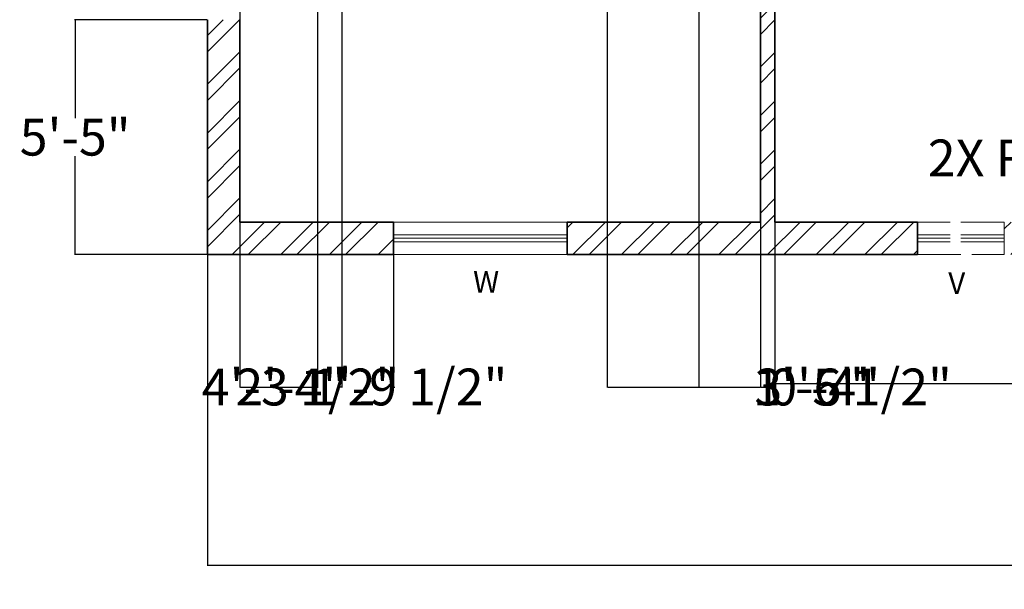
# Model space of a CAD drawing. Units: inches. Extents: x 1583 to 2239, y 1430 to 2174.
# Tile 1 of 5: x 1599 to 1871, y 1430 to 1588. Entities that reach past the tile are written whole.
import ezdxf

# ---------------------------------------------------------------- set-up
doc = ezdxf.new("R2010")
doc.units = ezdxf.units.IN
doc.linetypes.add('ACAD_ISO02W100', pattern=[15, 12, -3])
for name, color, linetype, lineweight in [('A-ANNO-DIMS', 2, 'Continuous', 18), ('A-ANNO-TEXT', 7, 'Continuous', 18), ('A-GLAZ-VENT', 6, 'ACAD_ISO02W100', 13), ('A-WALL-PATT', 252, 'Continuous', 13), ('WALL', 7, 'Continuous', 35), ('WINDOW', 160, 'Continuous', 18)]:
    doc.layers.add(name, color=color, linetype=linetype, lineweight=lineweight)
doc.styles.get("Standard").update_dxf_attribs({"font": 'arial.ttf'})
doc.dimstyles.get("Standard").update_dxf_attribs({"dimtxt": 10.18, "dimasz": 0.18, "dimexe": 0.18, "dimexo": 0.0625, "dimgap": 0.09, "dimtad": 0, "dimtih": 1, "dimtoh": 1, "dimdec": 0, "dimzin": 0, "dimdsep": 46, "dimlunit": 3, "dimtxsty": 'Standard', "dimcen": 0.09, "dimadec": 0, "dimazin": 0, "dimtfac": 1, "dimtdec": 0, "dimtofl": 0, "dimtmove": 0, "dimatfit": 3, "dimfxl": 1, "dimtolj": 1, "dimtzin": 0, "dimarcsym": 0})

# ---------------------------------------------------------------- blocks, each defined once
blk = doc.blocks.new('*D3')
at = {"layer": 'A-ANNO-DIMS', "color": 0, "lineweight": -2, "transparency": 16777216}
for p, q in [((1807.53, 1531.58), (1807.53, 1486.86)), ((2121.53, 1531.58), (2121.53, 1486.86)), ((1807.71, 1487.04), (1946.87, 1487.04)), ((2121.35, 1487.04), (1982.19, 1487.04))]:
    blk.add_line(p, q, dxfattribs=at)
at = {"layer": 'A-ANNO-DIMS', "color": 0, "transparency": 16777216}
for points in [[(1807.71, 1487.07), (1807.71, 1487.01), (1807.53, 1487.04)], [(2121.35, 1487.07), (2121.35, 1487.01), (2121.53, 1487.04)]]:
    blk.add_solid(points, dxfattribs=at)
at = {"layer": 'Defpoints', "color": 0, "transparency": 16777216}
for p in [(1807.53, 1531.64), (2121.53, 1531.64), (2121.53, 1487.04)]:
    blk.add_point(p, dxfattribs=at)
at = {"layer": 'A-ANNO-DIMS', "color": 0, "transparency": 16777216, "insert": (1964.53, 1487.04), "char_height": 10.18, "attachment_point": 5}
blk.add_mtext('\\A1;26\'-2"', dxfattribs=at)
blk = doc.blocks.new('*D9')
at = {"layer": 'A-ANNO-DIMS', "color": 0, "lineweight": -2, "transparency": 16777216}
for p, q in [((1650.53, 1522.58), (1650.53, 1436.63)), ((2130.53, 1522.58), (2130.53, 1436.63)), ((1650.71, 1436.81), (1881.6, 1436.81)), ((2130.35, 1436.81), (1899.47, 1436.81))]:
    blk.add_line(p, q, dxfattribs=at)
at = {"layer": 'A-ANNO-DIMS', "color": 0, "transparency": 16777216}
for points in [[(1650.71, 1436.84), (1650.71, 1436.78), (1650.53, 1436.81)], [(2130.35, 1436.84), (2130.35, 1436.78), (2130.53, 1436.81)]]:
    blk.add_solid(points, dxfattribs=at)
at = {"layer": 'Defpoints', "color": 0, "transparency": 16777216}
for p in [(1650.53, 1522.64), (2130.53, 1522.64), (2130.53, 1436.81)]:
    blk.add_point(p, dxfattribs=at)
at = {"layer": 'A-ANNO-DIMS', "color": 0, "transparency": 16777216, "insert": (1890.53, 1436.81), "char_height": 10.18, "attachment_point": 5}
blk.add_mtext("\\A1;40'", dxfattribs=at)
blk = doc.blocks.new('WIN-SASH-48IN')
for p, q in [((48, 2), (0, 2)), ((48, 1), (0, 1)), ((48, 0), (0, 0))]:
    blk.add_line(p, q)
blk = doc.blocks.new('VENT-GRILLE-24IN')
for p, q in [((24, 2), (0, 2)), ((24, 1), (0, 1)), ((24, 0), (0, 0))]:
    blk.add_line(p, q)
blk = doc.blocks.new('*D32')
at = {"layer": 'A-ANNO-DIMS', "color": 0, "lineweight": -2, "transparency": 16777216}
for p, q in [((1650.53, 1522.58), (1650.53, 1485.86)), ((1702.06, 1522.58), (1702.06, 1485.86)), ((1650.35, 1486.04), (1650.17, 1486.04)), ((1702.24, 1486.04), (1702.42, 1486.04))]:
    blk.add_line(p, q, dxfattribs=at)
at = {"layer": 'A-ANNO-DIMS', "color": 0, "transparency": 16777216}
for points in [[(1650.35, 1486.07), (1650.35, 1486.01), (1650.53, 1486.04)], [(1702.24, 1486.07), (1702.24, 1486.01), (1702.06, 1486.04)]]:
    blk.add_solid(points, dxfattribs=at)
at = {"layer": 'Defpoints', "color": 0, "transparency": 16777216}
for p in [(1650.53, 1522.64), (1702.06, 1522.64), (1702.06, 1486.04)]:
    blk.add_point(p, dxfattribs=at)
at = {"layer": 'A-ANNO-DIMS', "color": 0, "transparency": 16777216, "insert": (1676.29, 1486.04), "char_height": 10.18, "attachment_point": 5}
blk.add_mtext('\\A1;4\'-3 1/2"', dxfattribs=at)
blk = doc.blocks.new('*D36')
at = {"layer": 'A-ANNO-DIMS', "color": 0, "lineweight": -2, "transparency": 16777216}
for p, q in [((1650.47, 1587.56), (1613.75, 1587.56)), ((1613.93, 1587.38), (1613.93, 1560.37)), ((1613.93, 1522.82), (1613.93, 1549.83)), ((1650.47, 1522.64), (1613.75, 1522.64))]:
    blk.add_line(p, q, dxfattribs=at)
at = {"layer": 'A-ANNO-DIMS', "color": 0, "transparency": 16777216}
for points in [[(1613.9, 1587.38), (1613.96, 1587.38), (1613.93, 1587.56)], [(1613.9, 1522.82), (1613.96, 1522.82), (1613.93, 1522.64)]]:
    blk.add_solid(points, dxfattribs=at)
at = {"layer": 'Defpoints', "color": 0, "transparency": 16777216}
for p in [(1613.93, 1587.56), (1650.53, 1587.56), (1650.53, 1522.64)]:
    blk.add_point(p, dxfattribs=at)
at = {"layer": 'A-ANNO-DIMS', "color": 0, "transparency": 16777216, "insert": (1613.93, 1555.1), "char_height": 10.18, "attachment_point": 5}
blk.add_mtext('\\A1;5\'-5"', dxfattribs=at)
blk = doc.blocks.new('*D49')
at = {"layer": 'A-ANNO-DIMS', "color": 0, "lineweight": -2, "transparency": 16777216}
for p, q in [((1803.53, 1693.58), (1803.53, 1485.86)), ((1807.53, 1689.58), (1807.53, 1485.86)), ((1803.71, 1486.04), (1807.35, 1486.04)), ((1807.53, 1486.04), (1807.71, 1486.04))]:
    blk.add_line(p, q, dxfattribs=at)
at = {"layer": 'A-ANNO-DIMS', "color": 0, "transparency": 16777216}
for points in [[(1803.71, 1486.07), (1803.71, 1486.01), (1803.53, 1486.04)], [(1807.35, 1486.07), (1807.35, 1486.01), (1807.53, 1486.04)]]:
    blk.add_solid(points, dxfattribs=at)
at = {"layer": 'Defpoints', "color": 0, "transparency": 16777216}
for p in [(1803.53, 1693.64), (1807.53, 1689.64), (1807.53, 1486.04)]:
    blk.add_point(p, dxfattribs=at)
at = {"layer": 'A-ANNO-DIMS', "color": 0, "transparency": 16777216, "insert": (1821.33, 1486.04), "char_height": 10.18, "attachment_point": 5}
blk.add_mtext('\\A1;0\'-4"', dxfattribs=at)
blk = doc.blocks.new('*D53')
at = {"layer": 'A-ANNO-DIMS', "color": 0, "lineweight": -2, "transparency": 16777216}
for p, q in [((1659.53, 1693.58), (1659.53, 1485.86)), ((1687.68, 1693.86), (1687.68, 1485.86)), ((1659.71, 1486.04), (1659.9, 1486.04)), ((1687.5, 1486.04), (1687.31, 1486.04))]:
    blk.add_line(p, q, dxfattribs=at)
at = {"layer": 'A-ANNO-DIMS', "color": 0, "transparency": 16777216}
for points in [[(1659.71, 1486.07), (1659.71, 1486.01), (1659.53, 1486.04)], [(1687.5, 1486.07), (1687.5, 1486.01), (1687.68, 1486.04)]]:
    blk.add_solid(points, dxfattribs=at)
at = {"layer": 'Defpoints', "color": 0, "transparency": 16777216}
for p in [(1659.53, 1693.64), (1687.68, 1693.93), (1687.68, 1486.04)]:
    blk.add_point(p, dxfattribs=at)
at = {"layer": 'A-ANNO-DIMS', "color": 0, "transparency": 16777216, "insert": (1673.61, 1486.04), "char_height": 10.18, "attachment_point": 5}
blk.add_mtext('\\A1;2\'-4"', dxfattribs=at)
blk = doc.blocks.new('*D54')
at = {"layer": 'A-ANNO-DIMS', "color": 0, "lineweight": -2, "transparency": 16777216}
for p, q in [((1786.54, 1693.58), (1786.54, 1485.86)), ((1803.53, 1693.58), (1803.53, 1485.86)), ((1786.72, 1486.04), (1803.35, 1486.04)), ((1803.53, 1486.04), (1803.71, 1486.04))]:
    blk.add_line(p, q, dxfattribs=at)
at = {"layer": 'A-ANNO-DIMS', "color": 0, "transparency": 16777216}
for points in [[(1786.72, 1486.07), (1786.72, 1486.01), (1786.54, 1486.04)], [(1803.35, 1486.07), (1803.35, 1486.01), (1803.53, 1486.04)]]:
    blk.add_solid(points, dxfattribs=at)
at = {"layer": 'Defpoints', "color": 0, "transparency": 16777216}
for p in [(1786.54, 1693.64), (1803.53, 1693.64), (1803.53, 1486.04)]:
    blk.add_point(p, dxfattribs=at)
at = {"layer": 'A-ANNO-DIMS', "color": 0, "transparency": 16777216, "insert": (1816.85, 1486.04), "char_height": 10.18, "attachment_point": 5}
blk.add_mtext('\\A1;1\'-5"', dxfattribs=at)
blk = doc.blocks.new('*D59')
at = {"layer": 'A-ANNO-DIMS', "color": 0, "lineweight": -2, "transparency": 16777216}
for p, q in [((1659.53, 1801.58), (1659.53, 1485.86)), ((1681.03, 1801.01), (1681.03, 1485.86)), ((1659.71, 1486.04), (1680.85, 1486.04)), ((1681.03, 1486.04), (1681.21, 1486.04))]:
    blk.add_line(p, q, dxfattribs=at)
at = {"layer": 'A-ANNO-DIMS', "color": 0, "transparency": 16777216}
for points in [[(1659.71, 1486.07), (1659.71, 1486.01), (1659.53, 1486.04)], [(1680.85, 1486.07), (1680.85, 1486.01), (1681.03, 1486.04)]]:
    blk.add_solid(points, dxfattribs=at)
at = {"layer": 'Defpoints', "color": 0, "transparency": 16777216}
for p in [(1659.53, 1801.64), (1681.03, 1801.07), (1681.03, 1486.04)]:
    blk.add_point(p, dxfattribs=at)
at = {"layer": 'A-ANNO-DIMS', "color": 0, "transparency": 16777216, "insert": (1706.21, 1486.04), "char_height": 10.18, "attachment_point": 5}
blk.add_mtext('\\A1;1\'-9 1/2"', dxfattribs=at)
blk = doc.blocks.new('*D60')
at = {"layer": 'A-ANNO-DIMS', "color": 0, "lineweight": -2, "transparency": 16777216}
for p, q in [((1761.15, 1805.58), (1761.15, 1485.86)), ((1803.53, 1805.58), (1803.53, 1485.86)), ((1761.33, 1486.04), (1803.35, 1486.04)), ((1803.53, 1486.04), (1803.71, 1486.04))]:
    blk.add_line(p, q, dxfattribs=at)
at = {"layer": 'A-ANNO-DIMS', "color": 0, "transparency": 16777216}
for points in [[(1761.33, 1486.07), (1761.33, 1486.01), (1761.15, 1486.04)], [(1803.35, 1486.07), (1803.35, 1486.01), (1803.53, 1486.04)]]:
    blk.add_solid(points, dxfattribs=at)
at = {"layer": 'Defpoints', "color": 0, "transparency": 16777216}
for p in [(1761.15, 1805.64), (1803.53, 1805.64), (1803.53, 1486.04)]:
    blk.add_point(p, dxfattribs=at)
at = {"layer": 'A-ANNO-DIMS', "color": 0, "transparency": 16777216, "insert": (1829.19, 1486.04), "char_height": 10.18, "attachment_point": 5}
blk.add_mtext('\\A1;3\'-6 1/2"', dxfattribs=at)
blk = doc.blocks.new('*D63')
at = {"layer": 'A-ANNO-DIMS', "color": 0, "lineweight": -2, "transparency": 16777216}
for p, q in [((1916.32, 1549.35), (1916.5, 1549.35)), ((1916.5, 1549.35), (1925.71, 1540.14)), ((1941.32, 1524.44), (1941.5, 1524.44)), ((1941.41, 1524.35), (1941.41, 1524.53))]:
    blk.add_line(p, q, dxfattribs=at)
at = {"layer": 'A-ANNO-DIMS', "color": 0, "transparency": 16777216}
blk.add_solid([(1925.73, 1540.16), (1925.69, 1540.12), (1925.84, 1540.01)], dxfattribs=at)
at = {"layer": 'Defpoints', "color": 0, "transparency": 16777216}
for p in [(1925.84, 1540.01), (1941.41, 1524.44)]:
    blk.add_point(p, dxfattribs=at)
at = {"layer": 'A-ANNO-DIMS', "color": 0, "transparency": 16777216, "insert": (1882.85, 1549.35), "char_height": 10.18, "attachment_point": 5}
blk.add_mtext('\\A1;2X R1\'-10"', dxfattribs=at)

msp = doc.modelspace()

# ---------------------------------------------------------------- hatches: boundary and pattern name
at = {"layer": 'A-WALL-PATT'}
h = msp.add_hatch(dxfattribs=at)
h.set_pattern_fill('ANSI32', color=256)
h.paths.add_polyline_path([(1715.9, 2122.64), (1650.53, 2122.64), (1650.53, 1975.26), (1659.53, 1975.26), (1659.53, 1975.26), (1659.53, 2013.64), (1803.53, 2013.64), (1803.53, 1917.64), (1807.53, 1917.64), (1807.53, 2013.64), (1839.53, 2013.64), (1839.53, 2017.64), (1659.53, 2017.64), (1659.53, 2113.64), (1715.9, 2113.64)])
h.paths.add_polyline_path([(1893.86, 2122.64), (1763.9, 2122.64), (1763.9, 2113.64), (1875.53, 2113.64), (1875.53, 2013.64), (1879.53, 2013.64), (1879.53, 2037.64), (1909.53, 2037.64), (1909.53, 2041.64), (1879.53, 2041.64), (1879.53, 2113.64), (1893.86, 2113.64)])
h.paths.add_polyline_path([(1999.8, 2122.64), (1917.86, 2122.64), (1917.86, 2113.64), (1939.53, 2113.64), (1939.53, 2037.64), (1939.53, 1941.64), (1943.53, 1941.64), (1943.53, 2049.64), (2091.53, 2049.64), (2091.53, 2053.64), (1943.53, 2053.64), (1943.53, 2113.64), (1999.8, 2113.64)])
h.paths.add_polyline_path([(2130.53, 2122.64), (2023.8, 2122.64), (2023.8, 2113.64), (2121.53, 2113.64), (2121.53, 2049.64), (2121.53, 2013.82), (2130.53, 2013.82), (2130.53, 2013.82)])
h.paths.add_polyline_path([(2130.53, 1965.82), (2121.53, 1965.82), (2121.53, 1905.64), (1944.53, 1905.64), (1944.53, 1905.64), (1939.53, 1905.64), (1939.53, 1901.64), (2121.53, 1901.64), (2121.53, 1879.63), (2130.53, 1879.63)])
h.paths.add_polyline_path([(2130.53, 1855.63), (2121.53, 1855.63), (2121.53, 1817.64), (1939.53, 1817.64), (1939.53, 1729.64), (1943.53, 1729.64), (1943.53, 1813.64), (2121.53, 1813.64), (2121.53, 1780.2), (2130.53, 1780.2), (2130.53, 1780.2)])
h.paths.add_polyline_path([(2130.53, 1732.2), (2121.53, 1732.2), (2121.53, 1693.64), (1944.53, 1693.64), (1944.53, 1693.64), (1939.53, 1693.64), (1900.39, 1693.64), (1900.39, 1689.64), (2121.53, 1689.64), (2121.53, 1649.31), (2130.53, 1649.31), (2130.53, 1649.31)])
h.paths.add_polyline_path([(2130.53, 1601.31), (2121.53, 1601.31), (2121.53, 1531.64), (2056.46, 1531.64), (2056.46, 1522.64), (2130.53, 1522.64)])
h.paths.add_polyline_path([(2032.46, 1531.64), (1943.39, 1531.64), (1943.39, 1526.25), (1943.39, 1526.25), (1943.39, 1522.64), (2032.46, 1522.64)])
h.paths.add_polyline_path([(1895.39, 1531.64), (1871.02, 1531.64), (1871.02, 1522.64), (1895.39, 1522.64)])
h.paths.add_polyline_path([(1847.02, 1531.64), (1807.53, 1531.64), (1807.53, 1653.64), (1803.53, 1653.64), (1803.53, 1531.64), (1750.06, 1531.64), (1750.06, 1522.64), (1847.02, 1522.64)])
h.paths.add_polyline_path([(1702.06, 1531.64), (1659.53, 1531.64), (1659.53, 1587.56), (1650.53, 1587.56), (1650.53, 1522.64), (1702.06, 1522.64)])
h.paths.add_polyline_path([(1659.53, 1927.26), (1650.53, 1927.26), (1650.53, 1843.95), (1659.53, 1843.95), (1659.53, 1877.64)])
h.paths.add_polyline_path([(1659.53, 1801.64), (1807.53, 1801.64), (1807.53, 1881.64), (1689.53, 1881.64), (1689.53, 1877.64), (1803.53, 1877.64), (1803.53, 1805.64), (1659.53, 1805.64), (1659.53, 1819.95), (1650.53, 1819.95), (1650.53, 1766.08), (1659.53, 1766.08)])
h.paths.add_polyline_path([(1659.53, 1742.08), (1650.53, 1742.08), (1650.53, 1635.56), (1659.53, 1635.56), (1659.53, 1635.56), (1659.53, 1689.64), (1807.53, 1689.64), (1840.39, 1689.64), (1840.39, 1693.64), (1807.53, 1693.64), (1807.53, 1771.64), (1803.53, 1771.64), (1803.53, 1693.64), (1786.54, 1693.64), (1786.54, 1693.64), (1768.55, 1693.64), (1659.53, 1693.64), (1659.53, 1701.64)])

# ---------------------------------------------------------------- linework, layer by layer
at = {"layer": 'A-GLAZ-VENT'}
msp.add_lwpolyline([(1847.02, 1531.64), (1847.02, 1522.64), (1871.02, 1522.64), (1871.02, 1531.64)], close=True, dxfattribs=at)
at = {"layer": 'WALL'}
for p, q in [((1803.53, 1531.64), (1803.53, 1653.64)), ((1807.53, 1531.64), (1807.53, 1653.64)), ((1650.53, 1522.64), (1650.53, 1587.56)), ((1659.53, 1531.64), (1659.53, 1587.56)), ((1702.06, 1531.64), (1659.53, 1531.64)), ((1702.06, 1531.64), (1702.06, 1522.64)), ((1803.53, 1531.64), (1750.06, 1531.64)), ((1750.06, 1531.64), (1750.06, 1522.64)), ((1847.02, 1531.64), (1807.53, 1531.64)), ((1847.02, 1522.64), (1847.02, 1531.64)), ((1702.06, 1522.64), (1650.53, 1522.64)), ((1847.02, 1522.64), (1750.06, 1522.64))]:
    msp.add_line(p, q, dxfattribs=at)
at = {"layer": 'WINDOW'}
for p, q in [((1750.06, 1531.64), (1702.06, 1531.64)), ((1702.06, 1522.64), (1750.06, 1522.64))]:
    msp.add_line(p, q, dxfattribs=at)

# ---------------------------------------------------------------- block references
at = {"layer": 'A-GLAZ-VENT'}
msp.add_blockref('VENT-GRILLE-24IN', (1847.02, 1526.14), dxfattribs=at)
at = {"layer": 'WINDOW', "rotation": 180}
msp.add_blockref('WIN-SASH-48IN', (1750.06, 1528.14), dxfattribs=at)

# ---------------------------------------------------------------- texts
at = {"layer": 'A-ANNO-TEXT', "char_height": 6, "attachment_point": 1}
for s, insert in [('W', (1724.05, 1518.08)), ('V', (1855.51, 1517.77))]:
    msp.add_mtext_dynamic_manual_height_columns(s, width=236.3031, gutter_width=12.5, heights=[0], dxfattribs=dict(at, insert=insert))

# ---------------------------------------------------------------- dimensions: what is measured, and where the dimension line sits
at = {"layer": 'A-ANNO-DIMS'}
for base, p1, p2, override, picture, middle in [((1803.53, 1486.04), (1761.15, 1805.64), (1803.53, 1805.64), {"dimdec": 1, "dimlfac": 1, "dimrnd": 0, "dimzin": 1, "dimdsep": 46, "dimlunit": 4, "dimfrac": 2}, '*D60', (1829.19, 1486.04)), ((1681.03, 1486.04), (1659.53, 1801.64), (1681.03, 1801.07), {"dimdec": 1, "dimlfac": 1, "dimrnd": 0, "dimzin": 1, "dimdsep": 46, "dimlunit": 4, "dimfrac": 2}, '*D59', (1706.21, 1486.04)), ((1687.678, 1486.0388), (1659.532, 1693.6388), (1687.678, 1693.9271), {"dimdec": 1, "dimlfac": 1, "dimrnd": 0, "dimzin": 1, "dimdsep": 46, "dimlunit": 4, "dimfrac": 2}, '*D53', (1673.605, 1486.0388)), ((1803.53, 1486.04), (1786.54, 1693.64), (1803.53, 1693.64), {"dimdec": 1, "dimlfac": 1, "dimrnd": 0, "dimzin": 1, "dimdsep": 46, "dimlunit": 4, "dimfrac": 2}, '*D54', (1816.85, 1486.04)), ((1807.53, 1486.04), (1803.53, 1693.64), (1807.53, 1689.64), {"dimdec": 1, "dimlfac": 1, "dimrnd": 0, "dimzin": 1, "dimdsep": 46, "dimlunit": 4, "dimfrac": 2}, '*D49', (1821.33, 1486.04)), ((2121.53, 1487.04), (1807.53, 1531.64), (2121.53, 1531.64), {"dimclrd": 0, "dimclre": 0, "dimclrt": 0}, '*D3', (1964.53, 1487.04)), ((1702.06, 1486.04), (1650.53, 1522.64), (1702.06, 1522.64), {"dimdec": 1, "dimlfac": 1, "dimrnd": 0, "dimzin": 1, "dimdsep": 46, "dimlunit": 4, "dimfrac": 2}, '*D32', (1676.29, 1486.04)), ((2130.53, 1436.81), (1650.53, 1522.64), (2130.53, 1522.64), {"dimclrd": 0, "dimclre": 0, "dimclrt": 0}, '*D9', (1890.53, 1436.81))]:
    dim = msp.add_linear_dim(base=base, p1=p1, p2=p2, dimstyle='Standard', override=override, dxfattribs=at)
    dim.commit()
    dim.dimension.update_dxf_attribs({"geometry": picture, "text_midpoint": middle})
dim = msp.add_linear_dim(base=(1613.93, 1587.56), p1=(1650.53, 1522.64), p2=(1650.53, 1587.56), angle=90, dimstyle='Standard', override={"dimdec": 1, "dimlfac": 1, "dimrnd": 0, "dimzin": 1, "dimdsep": 46, "dimlunit": 4, "dimfrac": 2}, dxfattribs=at)
dim.commit()
dim.dimension.update_dxf_attribs({"geometry": '*D36', "text_midpoint": (1613.93, 1555.1)})
dim = msp.add_radius_dim(center=(1941.41, 1524.44), mpoint=(1925.84, 1540.01), text='2X <>', dimstyle='Standard', override={"dimdec": 1, "dimlfac": 1, "dimrnd": 0, "dimzin": 1, "dimdsep": 46, "dimlunit": 4, "dimfrac": 2}, dxfattribs=at)
dim.commit()
dim.dimension.update_dxf_attribs({"geometry": '*D63', "text_midpoint": (1882.85, 1549.35), "dimtype": 164})

doc.saveas('drawing.dxf')
